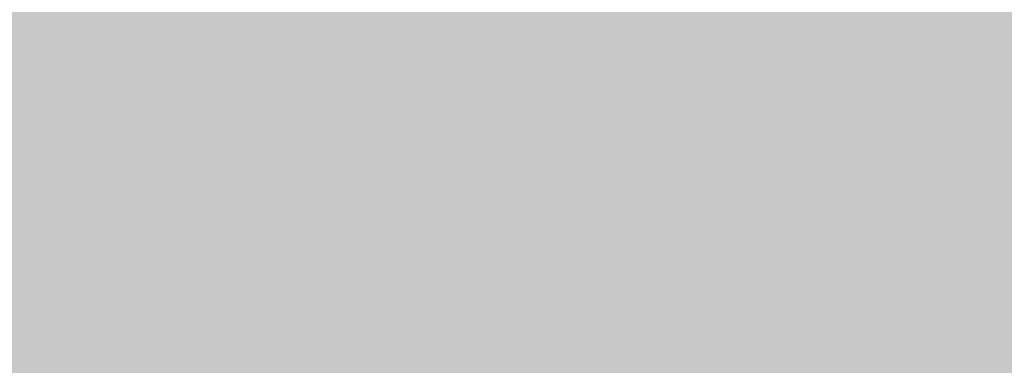
# Model space of a CAD drawing. Units: inches. Extents: x 2091 to 2899, y 967 to 2217.
# Tile 203 of 256: x 2203.18039 to 2203.25707, y 1152.27396 to 1152.30086. Entities that reach past the tile are written whole.
import ezdxf

# ---------------------------------------------------------------- set-up
doc = ezdxf.new("R2010")
doc.units = ezdxf.units.IN
doc.layers.add('A-WALL-PATT', color=141, linetype='Continuous', lineweight=13, true_color=0xadddf7)

msp = doc.modelspace()

# ---------------------------------------------------------------- hatches: boundary and pattern name
at = {"layer": 'A-WALL-PATT'}
h = msp.add_hatch(color=256, dxfattribs=at)
h.dxf.hatch_style = 1
h.paths.add_polyline_path([(2803.143603, 2050.919059), (2203.143603, 2050.919059), (2203.143603, 1090.919059), (2803.143603, 1090.919059)])
h.paths.add_polyline_path([(2635.79885, 1147.540465), (2674.524052, 1147.540465, 0.376086), (2678.529665, 1152.880202), (2678.529665, 1159.556473, 0.333335), (2674.524319, 1163.561846), (2674.524319, 1163.56185), (2674.524319, 1192.93439), (2635.805971, 1192.93439), (2597.087622, 1192.93439), (2597.087622, 1163.561846, 0.333335), (2593.082276, 1159.556473), (2593.082276, 1152.880202, 0.376086), (2597.087889, 1147.540465)], flags=0)
h.paths.add_polyline_path([(2436.010433, 1278.240778, 0.000483), (2435.952643, 1278.215027, -0.001328), (2435.935625, 1278.111693, -0.001711), (2436.11644, 1278.040758, 0.002185)], flags=0)
h.paths.add_polyline_path([(2794.143603, 1143.419059), (2794.143603, 1347.419059), (2543.370171, 1347.419059), (2543.370171, 1351.919059), (2794.143603, 1351.919059), (2794.143603, 1392.713555), (2793.947398, 1392.713555), (2793.947398, 1473.5369), (2794.143603, 1473.5369), (2794.143603, 1531.919059), (2650.143603, 1531.919059), (2650.143603, 1536.419059), (2794.143603, 1536.419059), (2794.143603, 1692.419059), (2609.375609, 1692.419059), (2609.375609, 1644.419059), (2604.875609, 1644.419059), (2604.875609, 1744.919059), (2609.375609, 1744.919059), (2609.375609, 1696.919059), (2794.143603, 1696.919059), (2794.143603, 1780.919059), (2609.643603, 1780.919059), (2493.875609, 1780.919059), (2493.875609, 1785.419059), (2609.643603, 1785.419059), (2794.143603, 1785.419059), (2794.143603, 1847.938821), (2793.951222, 1847.938821), (2793.951222, 1928.762166), (2794.143603, 1928.762166), (2794.143603, 1941.419059), (2614.143603, 1941.419059), (2614.143603, 1821.419059), (2609.643603, 1821.419059), (2609.643603, 1941.419059), (2392.143603, 1941.419059), (2392.143603, 1819.919059), (2387.643603, 1819.919059), (2387.643603, 1941.419059), (2212.143603, 1941.419059), (2212.143603, 1783.919059), (2392.143603, 1783.919059), (2392.143603, 1780.919059), (2212.143603, 1780.919059), (2212.143603, 1629.419059), (2387.643603, 1629.419059), (2387.643603, 1744.919059), (2392.143603, 1744.919059), (2392.143603, 1627.919059), (2317.143603, 1627.919059), (2317.143603, 1551.419059), (2317.143603, 1536.419059), (2459.383591, 1536.419059), (2459.383591, 1602.39648), (2463.883591, 1602.39648), (2463.883591, 1531.919059), (2456.643603, 1531.919059), (2456.643603, 1529.919059), (2452.143603, 1529.919059), (2452.143603, 1531.919059), (2312.643603, 1531.919059), (2312.643603, 1551.419059), (2306.143603, 1551.419059), (2306.143603, 1555.919059), (2308.143603, 1555.919059), (2308.143603, 1551.419059), (2312.643603, 1551.419059), (2312.643603, 1627.919059), (2212.143603, 1627.919059), (2212.143603, 1555.919059), (2270.143603, 1555.919059), (2270.143603, 1551.419059), (2212.143603, 1551.419059), (2212.143603, 1351.919059), (2272.143603, 1351.919059), (2272.143603, 1347.419059), (2212.143603, 1347.419059), (2212.143603, 1275.419059), (2308.143603, 1275.419059), (2308.143603, 1351.919059), (2452.143603, 1351.919059), (2452.143603, 1493.919059), (2456.643603, 1493.919059), (2456.643603, 1347.419059), (2312.643603, 1347.419059), (2312.643603, 1270.919059), (2212.143603, 1270.919059), (2212.143603, 1099.919059), (2281.237523, 1099.919059), (2282.871041, 1110.913803), (2282.008341, 1116.996603), (2278.557741, 1121.420403), (2268.205641, 1128.056203), (2272.087641, 1128.056203), (2273.812941, 1131.927003), (2279.420341, 1134.691903), (2285.027841, 1135.244903), (2287.615841, 1137.456803), (2288.047141, 1138.009803), (2289.341141, 1140.774703), (2291.066541, 1139.668703), (2292.360541, 1135.244903), (2295.379841, 1136.903803), (2296.242541, 1135.797903), (2297.105241, 1133.033003), (2300.124641, 1138.009803), (2303.143941, 1138.009803), (2304.437941, 1135.797903), (2303.143941, 1133.586003), (2306.594641, 1134.691903), (2307.888741, 1133.033003), (2310.908041, 1135.244903), (2313.927441, 1134.138903), (2315.62686, 1132.427102), (2308.320041, 1117.549603), (2290.203841, 1109.807903), (2288.909841, 1103.172103), (2289.272309, 1099.919059), (2434.918227, 1099.919059), (2431.593227, 1124.788059), (2429.930227, 1169.553059), (2430.927185, 1240.519694), (2435.658926, 1238.186126), (2437.135227, 1196.554059), (2438.798227, 1143.973059), (2442.678227, 1111.998059), (2446.558227, 1099.919059), (2794.143603, 1099.919059), (2794.143603, 1138.919059), (2548.032447, 1138.919059), (2548.032447, 1143.419059), (2548.032447, 1148.819059), (2546.668457, 1148.031559), (2528.685692, 1179.178622, 0.256256), (2512.032447, 1148.819059), (2512.032447, 1143.419059), (2512.032447, 1138.919059), (2507.532447, 1138.919059), (2507.532447, 1143.419059), (2507.532447, 1148.819059, 0.256256), (2490.879202, 1179.178622), (2472.896437, 1148.031559), (2471.532447, 1148.819059), (2471.532447, 1143.419059), (2467.032447, 1143.419059), (2467.032447, 1269.945786, 0.039061), (2460.909987, 1273.580059), (2467.032447, 1273.580059), (2467.032447, 1286.325364, 0.014511), (2465.216194, 1286.761905), (2467.032447, 1287.052576), (2467.032447, 1323.419059), (2471.532447, 1323.419059), (2471.532447, 1148.819059), (2489.532447, 1179.995973), (2490.896437, 1179.208473), (2490.879202, 1179.178622, -0.256256), (2507.532447, 1148.819059), (2507.532447, 1143.419059), (2512.032447, 1143.419059), (2512.032447, 1148.819059, -0.256256), (2528.685692, 1179.178622), (2528.668457, 1179.208473), (2530.032447, 1179.995973), (2548.032447, 1148.819059), (2548.032447, 1143.419059)], flags=16)
h.paths.add_polyline_path([(2607.768546, 1200.945083), (2607.768546, 1265.030625), (2597.087622, 1281.052011), (2619.784585, 1281.052011), (2627.795278, 1337.12686), (2635.79885, 1337.12686), (2643.816663, 1337.12686), (2651.827356, 1281.052011), (2674.524319, 1281.052011), (2663.843395, 1265.030625), (2663.843395, 1200.945083), (2635.805971, 1200.945083)], flags=0)
edge = h.paths.add_edge_path(flags=0)
edge.add_ellipse((13303.896215, 1272.998725), major_axis=(-10595.31304, 0.000001), ratio=0.842303870086, start_angle=0.6282372191, end_angle=0.6465540999, ccw=False)
edge.add_ellipse((2711.70045, 1156.852678), major_axis=(2.219769, 0), ratio=0.84230387, start_angle=111.535244, end_angle=180.628237, ccw=False)
edge.add_ellipse((13303.156292, 1272.998725), major_axis=(-10593.026306, 0), ratio=0.842303869544, start_angle=0.5282714718, end_angle=0.6465540971, ccw=False)
edge.add_line((2710.764596, 1175.333295), (2710.129986, 1175.333295))
edge.add_ellipse((2710.129986, 1176.579775), major_axis=(1.479846, 0), ratio=0.84230387, start_angle=180, end_angle=270, ccw=False)
edge.add_line((2708.65014, 1176.579775), (2708.65014, 1200.782914))
edge.add_ellipse((2710.129986, 1200.782914), major_axis=(1.479846, 0), ratio=0.84230387, start_angle=90, end_angle=180, ccw=False)
edge.add_line((2710.129986, 1202.029394), (2710.465075, 1202.029394))
edge.add_ellipse((13303.156292, 1272.998725), major_axis=(-10593.026306, 0), ratio=0.842303869544, start_angle=-0.0902290886, end_angle=0.3838667788, ccw=False)
edge.add_ellipse((2710.129986, 1290.927031), major_axis=(-1.479846, 0), ratio=0.84230387, start_angle=0, end_angle=90, ccw=False)
edge.add_line((2708.65014, 1290.927031), (2708.65014, 1315.13017))
edge.add_ellipse((2710.129986, 1315.13017), major_axis=(-1.479846, 0), ratio=0.84230387, start_angle=-90, end_angle=0, ccw=False)
edge.add_line((2710.129986, 1316.37665), (2710.706314, 1316.37665))
edge.add_ellipse((3238.40172, 1296.289566), major_axis=(528.234, 0), ratio=0.8423038695, start_angle=176.34957241, end_angle=177.82004969, ccw=False)
edge.add_ellipse((2775.063043, 1071.450696), major_axis=(313.307761, 0), ratio=0.8423038695, start_angle=102.12596555, end_angle=103.78052899, ccw=False)
edge.add_ellipse((2775.063043, 1078.305698), major_axis=(-305.302891, 0), ratio=0.8423038695, start_angle=-79.790461, end_angle=-77.55537271, ccw=False)
edge.add_ellipse((2695.141767, 1541.975383), major_axis=(-250.960216, 0), ratio=0.8423038695, start_angle=99.25656601, end_angle=102.55493264)
edge.add_line((2741.410326, 1334.214255), (2747.132545, 1337.378477))
edge.add_ellipse((2747.538616, 1336.857478), major_axis=(-0.739923, 0), ratio=0.8423039, start_angle=270, end_angle=307.93313, ccw=False)
edge.add_ellipse((2747.538616, 1336.857478), major_axis=(-0.739923, 0), ratio=0.8423039, start_angle=232.06687, end_angle=270, ccw=False)
edge.add_line((2747.944687, 1337.378477), (2753.666906, 1334.214255))
edge.add_ellipse((2799.935466, 1541.975383), major_axis=(250.960216, 0), ratio=0.8423038695, start_angle=257.44506736, end_angle=260.74343399)
edge.add_ellipse((2720.014189, 1078.305698), major_axis=(305.302891, 0), ratio=0.8423038695, start_angle=77.55537271, end_angle=79.790461, ccw=False)
edge.add_ellipse((2720.014189, 1071.450696), major_axis=(-313.307761, 0), ratio=0.8423038695, start_angle=256.21947101, end_angle=257.87403445, ccw=False)
edge.add_ellipse((2256.675512, 1296.289566), major_axis=(-528.234, 0), ratio=0.8423038695, start_angle=182.17995031, end_angle=183.65042759, ccw=False)
edge.add_line((2784.370918, 1316.37665), (2784.947247, 1316.37665))
edge.add_ellipse((2784.947247, 1315.13017), major_axis=(1.479846, 0), ratio=0.84230387, start_angle=0, end_angle=90, ccw=False)
edge.add_line((2786.427093, 1315.13017), (2786.427093, 1290.927031))
edge.add_ellipse((2784.947247, 1290.927031), major_axis=(1.479846, 0), ratio=0.84230387, start_angle=270, end_angle=360, ccw=False)
edge.add_ellipse((-7808.07906, 1272.998725), major_axis=(10593.026306, 0), ratio=0.842303869544, start_angle=-0.3838667788, end_angle=0.0902290886, ccw=False)
edge.add_line((2784.612157, 1202.029394), (2784.947247, 1202.029394))
edge.add_ellipse((2784.947247, 1200.782914), major_axis=(1.479846, 0), ratio=0.84230387, start_angle=0, end_angle=90, ccw=False)
edge.add_line((2786.427093, 1200.782914), (2786.427093, 1176.579775))
edge.add_ellipse((2784.947247, 1176.579775), major_axis=(-1.479846, 0), ratio=0.84230387, start_angle=90, end_angle=180, ccw=False)
edge.add_line((2784.947247, 1175.333295), (2784.312636, 1175.333295))
edge.add_ellipse((-7808.07906, 1272.998725), major_axis=(10593.026306, 0), ratio=0.842303869544, start_angle=-0.6186431963, end_angle=-0.5282714718, ccw=False)
edge.add_ellipse((2783.376783, 1156.852678), major_axis=(-2.219769, 0), ratio=0.84230387, start_angle=179.371763, end_angle=248.464757, ccw=False)
edge.add_ellipse((-7808.818983, 1272.998725), major_axis=(-10595.31304, 0.000004), ratio=0.842303865762, start_angle=179.3534459226, end_angle=179.3717628034, ccw=False)
edge.add_ellipse((2780.297303, 1153.500793), major_axis=(-5.246426, 0), ratio=0.84230387, start_angle=90, end_angle=179.353446, ccw=False)
edge.add_line((2780.297303, 1149.081708), (2714.77993, 1149.081708))
edge.add_ellipse((2714.77993, 1153.500793), major_axis=(5.246426, 0), ratio=0.84230387, start_angle=180.646554, end_angle=270, ccw=False)
edge = h.paths.add_edge_path(flags=0)
edge.add_line((2718.187367, 1151.007833), (2718.187367, 1170.472364))
edge.add_ellipse((2721.14706, 1170.472364), major_axis=(-2.959692, 0), ratio=0.84230387, start_angle=-90, end_angle=0, ccw=False)
edge.add_line((2721.14706, 1172.965324), (2773.930173, 1172.965324))
edge.add_ellipse((2773.930173, 1170.472364), major_axis=(-2.959692, 0), ratio=0.84230387, start_angle=180, end_angle=270, ccw=False)
edge.add_line((2776.889865, 1170.472364), (2776.889865, 1151.007833))
edge.add_line((2776.889865, 1151.007833), (2718.187367, 1151.007833))
edge = h.paths.add_edge_path(flags=0)
edge.add_line((2718.187367, 1180.23415), (2718.187367, 1199.057834))
edge.add_ellipse((2747.538616, 1320.39864), major_axis=(147.017924, 0), ratio=0.8423038695, start_angle=256.40186531, end_angle=283.59813469)
edge.add_line((2776.889865, 1199.057834), (2776.889865, 1180.23415))
edge.add_ellipse((2747.538616, 1301.574956), major_axis=(147.017924, 0), ratio=0.8423038695, start_angle=256.40186531, end_angle=283.59813469, ccw=False)
edge = h.paths.add_edge_path(flags=0)
edge.add_ellipse((13303.156292, 1272.998725), major_axis=(-10591.54646, 0), ratio=0.842303869555, start_angle=0.0555943135, end_angle=0.3777641939, ccw=False)
edge.add_line((2711.616859, 1262.72171), (2715.667408, 1249.495396))
edge.add_ellipse((6413.891963, 1241.691919), major_axis=(-3698.236159, 0), ratio=0.84230386955, start_angle=-0.120897369, end_angle=0.364076349)
edge.add_line((2715.761038, 1218.192455), (2711.934307, 1203.167361))
edge = h.paths.add_edge_path(flags=0)
edge.add_line((2718.187367, 1251.074566), (2716.002485, 1267.450435))
edge.add_ellipse((2742.151175, 1202.18954), major_axis=(81.772585, 0), ratio=0.84230387, start_angle=94.27742096, end_angle=111.8349538, ccw=False)
edge.add_line((2737.009748, 1270.930626), (2758.067484, 1270.930626))
edge.add_ellipse((2752.926058, 1202.18954), major_axis=(81.772585, 0), ratio=0.84230387, start_angle=68.1650462, end_angle=85.72257904, ccw=False)
edge.add_line((2779.074747, 1267.450435), (2776.889865, 1251.074566))
edge.add_ellipse((2750.338059, 1187.885356), major_axis=(79.579664, 0), ratio=0.84230387, start_angle=67.20808512, end_angle=85.1299304)
edge.add_line((2756.034656, 1254.743656), (2739.042576, 1254.743656))
edge.add_ellipse((2744.739174, 1187.885356), major_axis=(79.579664, 0), ratio=0.84230387, start_angle=94.8700696, end_angle=112.79191488)
edge = h.paths.add_edge_path(flags=0)
edge.add_line((2783.142926, 1203.167361), (2779.316194, 1218.192455))
edge.add_ellipse((-918.81473, 1241.691919), major_axis=(3698.236159, 0), ratio=0.84230386955, start_angle=-0.364076349, end_angle=0.120897369)
edge.add_line((2779.409825, 1249.495396), (2783.460373, 1262.72171))
edge.add_ellipse((-7808.07906, 1272.998725), major_axis=(-10591.54646, 0), ratio=0.84230386954, start_angle=179.6222358061, end_angle=179.9444056865, ccw=False)
edge = h.paths.add_edge_path(flags=0)
edge.add_ellipse((2734.200892, 1286.69044), major_axis=(-0.356609, 6.340078), ratio=0.60383358, start_angle=89.0020143, end_angle=253.657408, ccw=False)
edge.add_line((2730.369001, 1286.541806), (2730.369001, 1301.35198))
edge.add_line((2730.369001, 1301.35198), (2735.913311, 1305.214803))
edge.add_ellipse((2736.384917, 1304.734561), major_axis=(0.739923, 0), ratio=0.8423039, start_angle=90, end_angle=134.480211, ccw=False)
edge.add_line((2736.384917, 1305.357801), (2738.032783, 1305.357801))
edge.add_line((2738.032783, 1305.357801), (2738.032783, 1307.707927))
edge.add_ellipse((2794.201642, 1307.707927), major_axis=(56.168859, 0), ratio=0.84230387, start_angle=150.5614304, end_angle=180, ccw=False)
edge.add_ellipse((2700.875591, 1307.707927), major_axis=(-56.168859, 0), ratio=0.84230387, start_angle=180, end_angle=209.4385696, ccw=False)
edge.add_line((2757.04445, 1307.707927), (2757.04445, 1305.357801))
edge.add_line((2757.04445, 1305.357801), (2758.692316, 1305.357801))
edge.add_ellipse((2758.692316, 1304.734561), major_axis=(-0.739923, 0), ratio=0.8423039, start_angle=225.519789, end_angle=270, ccw=False)
edge.add_line((2759.163922, 1305.214803), (2764.708231, 1301.35198))
edge.add_line((2764.708231, 1301.35198), (2764.708231, 1286.541806))
edge.add_ellipse((2760.87634, 1286.69044), major_axis=(0.356609, 6.340078), ratio=0.60383358, start_angle=106.342592, end_angle=270.9979857, ccw=False)
edge.add_line((2757.04445, 1285.79709), (2757.04445, 1307.707927))
edge.add_ellipse((2700.875591, 1307.707927), major_axis=(-56.168859, 0), ratio=0.84230387, start_angle=180, end_angle=209.4385696)
edge.add_ellipse((2794.201642, 1307.707927), major_axis=(56.168859, 0), ratio=0.84230387, start_angle=150.5614304, end_angle=180)
edge.add_line((2738.032783, 1307.707927), (2738.032783, 1285.79709))
h.paths.add_polyline_path([(2417.812273, 1104.449704), (2413.492273, 1102.529704), (2410.612273, 1103.969704), (2409.172273, 1106.369704), (2407.252273, 1107.329704), (2406.292273, 1109.729704), (2405.332273, 1114.049704), (2405.332273, 1117.889704), (2406.292273, 1120.129704), (2407.252273, 1119.809704), (2408.848322, 1118.327658), (2410.173945, 1119.42417), (2410.211273, 1120.405704), (2411.040731, 1121.419054), (2410.699273, 1119.858704), (2410.173945, 1119.42417), (2410.088452, 1117.176109), (2411.132836, 1116.206324), (2413.972273, 1119.329704), (2416.852273, 1120.769704), (2416.869721, 1120.798784), (2417.035071, 1119.405116), (2417.896213, 1118.143384), (2418.292273, 1118.369704), (2419.544447, 1120.039269), (2419.360915, 1118.387487), (2419.032108, 1119.356151), (2418.398939, 1118.511926), (2419.252273, 1114.529704), (2418.794091, 1107.198795)], flags=0)
h.paths.add_polyline_path([(2508.870171, 1347.419059), (2508.370171, 1347.419059), (2508.370171, 1351.919059), (2508.870171, 1351.919059)], flags=0)
h.paths.add_polyline_path([(2473.370171, 1347.419059), (2472.370171, 1347.419059), (2467.870171, 1347.419059), (2467.870171, 1455.419059), (2472.370171, 1455.419059), (2472.370171, 1352.419059), (2473.370171, 1352.419059)], flags=0)
h.paths.add_polyline_path([(2352.106244, 1217.446197), (2349.226244, 1218.886197), (2347.786244, 1221.286197), (2345.866244, 1222.246197), (2344.906244, 1224.646197), (2343.946244, 1228.966197), (2343.946244, 1232.806197), (2344.906244, 1235.046197), (2345.866244, 1234.726197), (2347.462293, 1233.244152), (2348.787916, 1234.340663), (2348.825244, 1235.322197), (2349.654702, 1236.335547), (2349.313244, 1234.775197), (2348.787916, 1234.340663), (2348.702423, 1232.092603), (2349.746807, 1231.122817), (2352.586244, 1234.246197), (2355.466244, 1235.686197), (2355.483692, 1235.715277), (2355.649043, 1234.321609), (2356.510185, 1233.059877), (2356.906244, 1233.286197), (2358.158418, 1234.955762), (2357.974887, 1233.30398), (2357.646079, 1234.272644), (2357.012911, 1233.428419), (2357.866244, 1229.446197), (2357.408062, 1222.115288), (2356.426244, 1219.366197)], flags=0)
h.paths.add_polyline_path([(2348.2968, 1112.22442), (2347.0138, 1112.31042), (2345.5298, 1114.12742), (2345.7318, 1115.85842), (2346.8118, 1116.98242), (2346.8118, 1114.64642), (2345.8668, 1114.21442), (2346.8798, 1114.30042)], flags=0)
h.paths.add_polyline_path([(2347.0138, 1110.92642), (2346.2718, 1110.49342), (2346.6098, 1111.18642)], flags=0)
h.paths.add_polyline_path([(2345.8668, 1118.19442), (2345.5298, 1117.32942), (2343.7078, 1118.02142), (2344.3828, 1118.62642)], flags=0)
h.paths.add_polyline_path([(2346.6768, 1109.28242), (2346.0698, 1108.07142), (2345.8668, 1110.06142)], flags=0)
h.paths.add_polyline_path([(2345.0568, 1119.75142), (2343.6398, 1119.75142), (2343.9778, 1121.13542)], flags=0)
h.paths.add_polyline_path([(2345.2598, 1116.55042), (2345.1248, 1115.85842), (2344.9218, 1115.68542), (2344.7198, 1116.37742)], flags=0)
h.paths.add_polyline_path([(2345.6648, 1112.31042), (2345.4618, 1111.53242), (2344.0448, 1111.96442), (2344.6518, 1112.57042)], flags=0)
h.paths.add_polyline_path([(2345.1918, 1113.34942), (2344.4498, 1113.86842), (2344.7198, 1114.38742)], flags=0)
h.paths.add_polyline_path([(2344.6518, 1116.80942), (2344.1798, 1115.68542), (2344.6518, 1115.33942), (2343.9098, 1114.90642), (2343.0328, 1115.94442), (2343.6398, 1116.46342)], flags=0)
h.paths.add_polyline_path([(2345.8668, 1106.68642), (2344.9898, 1105.56242), (2344.5168, 1106.60042)], flags=0)
h.paths.add_polyline_path([(2344.8548, 1110.06142), (2344.5168, 1109.28242), (2344.1128, 1109.71542)], flags=0)
h.paths.add_polyline_path([(2344.0448, 1113.52242), (2343.4378, 1113.08942), (2342.7628, 1113.95442)], flags=0)
h.paths.add_polyline_path([(2344.3148, 1111.01242), (2342.9648, 1110.32042), (2342.9648, 1111.09942)], flags=0)
h.paths.add_polyline_path([(2345.1248, 1104.69742), (2344.5848, 1103.74542), (2344.4498, 1104.26442)], flags=0)
h.paths.add_polyline_path([(2342.8298, 1121.22242), (2341.7498, 1120.53042), (2340.5358, 1121.04942), (2340.1308, 1121.82842), (2340.6708, 1122.95242), (2341.1428, 1121.82842), (2341.6148, 1122.00142)], flags=0)
h.paths.add_polyline_path([(2342.9648, 1119.75142), (2343.0328, 1118.45342), (2342.0878, 1118.02142), (2342.0198, 1119.49142)], flags=0)
h.paths.add_polyline_path([(2342.6948, 1116.89642), (2341.9528, 1116.63642), (2342.0198, 1117.32942)], flags=0)
h.paths.add_polyline_path([(2343.0328, 1112.22442), (2342.0198, 1111.79142), (2341.5478, 1112.22442), (2342.3578, 1113.34942)], flags=0)
h.paths.add_polyline_path([(2343.7748, 1104.43742), (2342.6278, 1102.88042), (2342.6948, 1104.61042), (2343.4378, 1105.12942)], flags=0)
h.paths.add_polyline_path([(2342.0198, 1115.07942), (2340.8058, 1115.51242), (2340.9408, 1116.37742)], flags=0)
h.paths.add_polyline_path([(2341.4808, 1120.09742), (2341.4808, 1119.40542), (2341.0758, 1119.57842), (2341.1428, 1120.09742)], flags=0)
h.paths.add_polyline_path([(2341.8178, 1114.47342), (2340.9408, 1113.08942), (2340.8058, 1114.56042)], flags=0)
h.paths.add_polyline_path([(2341.1428, 1118.54042), (2340.9408, 1116.98242), (2339.0508, 1117.67542), (2339.0508, 1118.62642)], flags=0)
h.paths.add_polyline_path([(2342.6948, 1101.66842), (2341.9528, 1101.84142), (2342.5598, 1102.36142)], flags=0)
h.paths.add_polyline_path([(2340.3328, 1119.66542), (2338.4438, 1119.57842), (2337.9038, 1120.35742), (2339.6578, 1120.61642)], flags=0)
h.paths.add_polyline_path([(2340.3328, 1115.33942), (2340.0628, 1113.69542), (2339.3878, 1115.33942)], flags=0)
h.paths.add_polyline_path([(2341.8178, 1103.83142), (2341.5478, 1102.88042), (2341.1428, 1103.65842)], flags=0)
h.paths.add_polyline_path([(2339.0508, 1122.86642), (2337.2958, 1121.82842), (2337.0938, 1123.12542), (2337.7688, 1123.81842)], flags=0)
h.paths.add_polyline_path([(2339.1178, 1121.74142), (2338.8478, 1121.22242), (2338.1738, 1121.04942), (2338.3758, 1121.56842)], flags=0)
h.paths.add_polyline_path([(2339.1858, 1119.31942), (2338.6458, 1118.71342), (2338.2408, 1118.10742), (2338.2408, 1118.88642)], flags=0)
h.paths.add_polyline_path([(2341.1428, 1101.92842), (2340.6028, 1101.23642), (2340.0628, 1101.84142), (2340.6028, 1102.36142)], flags=0)
h.paths.add_polyline_path([(2337.6338, 1117.76142), (2336.6208, 1118.28042), (2337.2958, 1118.97242)], flags=0)
h.paths.add_polyline_path([(2336.8238, 1119.57842), (2334.7988, 1118.97242), (2335.2038, 1120.35742), (2336.5538, 1120.87642)], flags=0)
h.paths.add_polyline_path([(2339.1178, 1100.45742), (2337.3638, 1100.54342), (2336.7558, 1101.23642)], flags=0)
h.paths.add_polyline_path([(2336.3508, 1122.43342), (2336.0138, 1121.91442), (2334.9338, 1122.43342), (2334.5288, 1123.47142), (2335.7438, 1122.77942)], flags=0)
h.paths.add_polyline_path([(2334.7318, 1120.87642), (2334.2588, 1120.35742), (2334.0568, 1120.78942), (2334.5968, 1121.30842)], flags=0)
h.paths.add_polyline_path([(2334.4618, 1122.17442), (2332.5718, 1121.30842), (2331.3568, 1122.17442), (2332.0998, 1122.86642)], flags=0)
h.paths.add_polyline_path([(2334.2588, 1118.54042), (2333.3818, 1118.45342), (2333.6518, 1119.31942)], flags=0)
h.paths.add_polyline_path([(2335.5418, 1102.27442), (2334.1918, 1102.62042), (2335.2718, 1103.31242)], flags=0)
h.paths.add_polyline_path([(2332.7068, 1119.66542), (2331.6948, 1120.44342), (2332.5048, 1120.78942)], flags=0)
h.paths.add_polyline_path([(2334.7318, 1101.14942), (2333.5168, 1101.58242), (2333.9888, 1101.75542)], flags=0)
h.paths.add_polyline_path([(2332.6398, 1116.63642), (2331.0868, 1116.29042), (2331.9648, 1118.19442)], flags=0)
h.paths.add_polyline_path([(2330.7498, 1121.56842), (2330.2768, 1120.27042), (2328.5228, 1119.31942), (2328.9948, 1121.04942)], flags=0)
h.paths.add_polyline_path([(2330.7498, 1118.62642), (2330.0078, 1117.50242), (2329.8728, 1118.02142)], flags=0)
h.paths.add_polyline_path([(2332.0998, 1102.36142), (2330.5468, 1102.01442), (2331.6948, 1102.96642)], flags=0)
h.paths.add_polyline_path([(2329.5348, 1113.60842), (2329.0628, 1112.31042), (2328.5898, 1113.34942)], flags=0)
h.paths.add_polyline_path([(2328.3878, 1117.84842), (2327.5098, 1116.55042), (2327.1728, 1117.76142)], flags=0)
h.paths.add_polyline_path([(2329.7378, 1106.51342), (2329.5348, 1105.30242), (2328.2528, 1106.08142)], flags=0)
h.paths.add_polyline_path([(2328.6578, 1114.38742), (2328.0498, 1114.12742), (2328.3198, 1114.90642)], flags=0)
h.paths.add_polyline_path([(2328.3198, 1112.22442), (2327.1058, 1112.13742), (2326.7008, 1112.65642)], flags=0)
h.paths.add_polyline_path([(2326.9028, 1115.25242), (2326.7008, 1114.12742), (2325.2158, 1113.60842), (2326.0928, 1115.33942)], flags=0)
h.paths.add_polyline_path([(2326.6328, 1108.33042), (2326.0928, 1107.37942), (2325.8908, 1108.50342), (2326.4978, 1109.10942)], flags=0)
h.paths.add_polyline_path([(2615.143603, 1531.919059), (2609.643603, 1531.919059), (2609.643603, 1620.419059), (2614.143603, 1620.419059), (2614.143603, 1536.419059), (2615.143603, 1536.419059)], flags=0)
h.paths.add_polyline_path([(2545.143603, 1563.419059), (2464.143603, 1563.419059), (2464.143603, 1632.419059), (2509.143603, 1632.419059), (2509.143603, 1627.919059), (2509.143603, 1603.919059), (2468.643603, 1603.919059), (2468.643603, 1567.919059), (2540.643603, 1567.919059), (2540.643603, 1591.919059), (2545.143603, 1591.919059)], flags=0)
h.paths.add_polyline_path([(2388.969048, 1549.985735), (2357.434181, 1549.985735), (2357.434181, 1623.360778), (2399.362777, 1623.360778), (2435.689465, 1623.360778), (2435.592547, 1602.559273), (2435.592547, 1602.39648), (2388.969048, 1602.39648)], flags=0)
h.paths.add_polyline_path([(2388.880628, 1555.809151), (2374.904429, 1555.809151), (2374.904429, 1600.571564), (2374.904429, 1615.457645), (2406.350877, 1615.457645), (2406.350877, 1618.939431), (2412.174293, 1615.457645), (2406.350877, 1611.97586), (2406.350877, 1615.457645), (2388.880628, 1615.457645)], flags=0)
h.paths.add_polyline_path([(2568.875609, 1644.419059), (2453.375609, 1644.419059), (2453.375609, 1785.419059), (2457.875609, 1785.419059), (2457.875609, 1648.919059), (2568.875609, 1648.919059)], flags=0)
h.paths.add_polyline_path([(2212.143603, 1945.919059), (2212.143603, 2041.919059), (2794.143603, 2041.919059), (2794.143603, 1945.919059)], flags=16)
h.paths.add_polyline_path([(2271.082728, 1964.317238), (2776.852968, 1964.317238), (2776.852968, 2037.169623), (2271.082728, 2037.169623)], flags=8)
h.paths.add_polyline_path([(2380.649285, 1536.824144), (2461.040809, 1536.824144), (2461.040809, 1554.652587), (2380.649285, 1554.652587)], flags=8)
h.paths.add_polyline_path([(2240.755709, 1609.725451), (2309.185829, 1609.725451), (2309.185829, 1617.698204), (2240.755709, 1617.698204)], flags=8)
h.paths.add_polyline_path([(2212.677255, 1313.504102), (2282.59152, 1313.504102), (2282.59152, 1322.745239), (2212.677255, 1322.745239)], flags=8)
h.paths.add_polyline_path([(2457.111976, 1114.778574), (2558.481581, 1114.778574), (2558.481581, 1142.219682), (2457.111976, 1142.219682)], flags=8)
h.paths.add_polyline_path([(2473.442337, 1273.010067), (2604.641226, 1273.010067), (2604.641226, 1318.346935), (2473.442337, 1318.346935)], flags=8)
h.paths.add_polyline_path([(2638.876302, 1626.977432), (2684.250367, 1627.976738), (2684.038483, 1637.597494), (2638.664417, 1636.598188)], flags=8)
h.paths.add_polyline_path([(2537.590554, 1453.793447), (2628.389547, 1453.793447), (2628.389547, 1475.344811), (2537.590554, 1475.344811)], flags=8)
h.paths.add_polyline_path([(2504.137638, 1714.632397), (2554.647187, 1714.632397), (2554.647187, 1730.237712), (2504.137638, 1730.237712)], flags=8)
h.paths.add_polyline_path([(2487.501181, 1575.651872), (2535.097121, 1575.651872), (2535.097121, 1598.377646), (2487.501181, 1598.377646)], flags=8)
h.paths.add_polyline_path([(2709.0994, 1735.710278), (2740.016601, 1735.710278), (2740.016601, 1749.937641), (2709.0994, 1749.937641)], flags=8)
h.paths.add_polyline_path([(2442.438424, 1792.171657), (2564.728835, 1792.171657), (2564.728835, 1842.000163), (2442.438424, 1842.000163)], flags=8)
h.paths.add_polyline_path([(2655.815801, 1809.644076), (2789.520142, 1806.693796), (2790.084977, 1832.291638), (2656.380635, 1835.241918)], flags=8)
h.paths.add_polyline_path([(2234.842697, 1797.720143), (2368.592851, 1794.768852), (2369.160718, 1820.504132), (2235.410564, 1823.455423)], flags=8)
h.paths.add_polyline_path([(2245.138466, 1644.006335), (2398.427733, 1640.6239), (2398.994842, 1666.32482), (2245.705575, 1669.707255)], flags=8)
h.paths.add_polyline_path([(2306.142847, 1431.168519), (2413.768314, 1428.793687), (2414.333148, 1454.391529), (2306.707682, 1456.76636)], flags=8)
h.paths.add_polyline_path([(2306.834582, 1458.233145), (2393.380484, 1456.323449), (2393.932808, 1481.354358), (2307.386907, 1483.264054)], flags=8)

doc.saveas('drawing.dxf')
